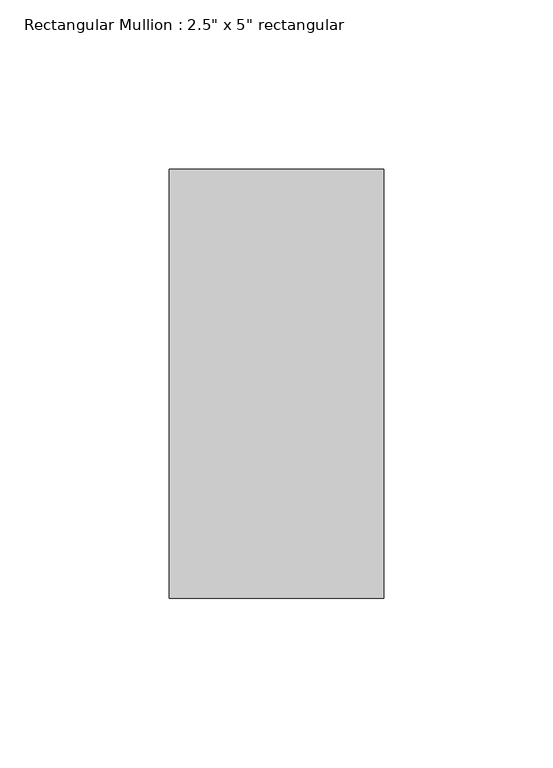
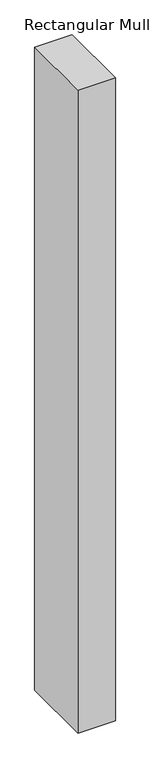
"""IFC4 building model written with IfcOpenShell, lengths in millimetres: member geometry."""

from ifc_helpers import new_model, si_unit, frame, origin, place, context, project, spatial, polyline, outline, extrude, source, transform, mapped, element, save


def member_49b1bc66(model_context):
    return source(origin(), model_context, "Body", "SweptSolid", [
        extrude(outline(polyline([(31.75, 63.5), (31.75, -63.5), (-31.75, -63.5), (-31.75, 63.5), (31.75, 63.5)])), frame((0.0, 0.0, -1153.7949999), z_axis=(0.0, 0.0, 1.0), x_axis=(1.0, 0.0, 0.0)), (0.0, 0.0, 1.0), 1153.7949999),
    ])


if __name__ == "__main__":
    model = new_model("IFC4")
    model_context = context("Model", 3, world=origin())
    ifc_project = project(units=[si_unit("LENGTHUNIT", "METRE", prefix="MILLI")], contexts=[model_context])
    site = spatial("IfcSite", under=ifc_project)
    building = spatial("IfcBuilding", under=site)
    placement = place(None, origin())
    member_shape = member_49b1bc66(model_context)
    element("IfcMember", 1, ObjectType="Rectangular Mullion : 2.5\" x 5\" rectangular", at=placement, inside=building, context=model_context, shape_type="MappedRepresentation", body=[
        mapped(member_shape, transform((0.0, 0.0, 0.0), x_axis=(1.0, 0.0, 0.0), y_axis=(0.0, 1.0, 0.0), z_axis=(0.0, 0.0, 1.0))),
    ])
    save(model, "model.ifc")

# Revit data of these elements
# Type "Rectangular Mullion : 2.5\" x 5\" rectangular"
#   built-in parameter 1007304 = 0.416667 (stored number, unit not read)
#   built-in parameter 1007301 = 0.104167 (stored number, unit not read)
#   built-in parameter 1007300 = 0.104167 (stored number, unit not read)
# Element 1 (IfcMember, "Rectangular Mullion : 2.5\" x 5\" rectangular")
#   Materials on its faces: "Aluminum"
# Materials
#   "Aluminum": class "Metal", colour RGB 247 247 247, transparency 0, Description = "Aluminum 6061", Cost = 0
